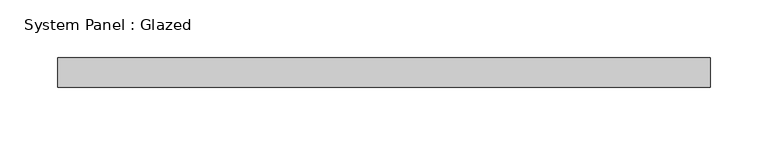
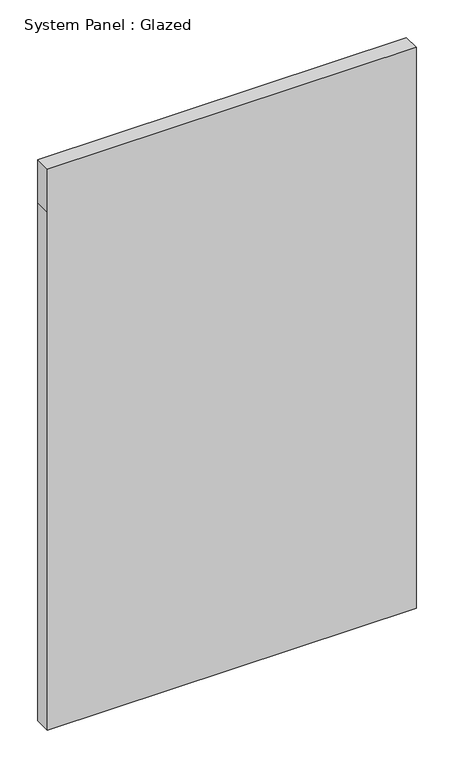
"""IFC4 building model written with IfcOpenShell, lengths in millimetres: plate geometry, System Panel : Glazed."""

from ifc_helpers import new_model, si_unit, frame, origin, place, context, project, spatial, polyline, outline, extrude, source, transform, mapped, element, save


def system_panel_glazed_cdc3472a(model_context):
    return source(origin(), model_context, "Body", "SweptSolid", [
        extrude(outline(polyline([(0.0, -282.575), (0.0, 282.575), (839.0301773, 282.575), (908.8801773, 282.575), (908.8801773, -282.575), (839.0301773, -282.575), (0.0, -282.575)])), frame((0.0, 19.05, 0.0), z_axis=(0.0, 1.0, 0.0), x_axis=(0.0, 0.0, 1.0)), (0.0, 0.0, 1.0), 25.4),
    ])


if __name__ == "__main__":
    model = new_model("IFC4")
    model_context = context("Model", 3, world=origin())
    ifc_project = project(units=[si_unit("LENGTHUNIT", "METRE", prefix="MILLI")], contexts=[model_context])
    site = spatial("IfcSite", under=ifc_project)
    building = spatial("IfcBuilding", under=site)
    placement = place(None, origin())
    system_panel_glazed_shape = system_panel_glazed_cdc3472a(model_context)
    element("IfcPlate", 1, ObjectType="System Panel : Glazed", at=placement, inside=building, context=model_context, shape_type="MappedRepresentation", body=[
        mapped(system_panel_glazed_shape, transform((0.0, 0.0, 0.0), x_axis=(1.0, 0.0, 0.0), y_axis=(0.0, 1.0, 0.0), z_axis=(0.0, 0.0, 1.0))),
    ])
    save(model, "model.ifc")

# Revit data of these elements
# Type "System Panel : Glazed"
#   Construction Type Id = "GSP4R"
#   Analytic Construction = "1/8 in Pilkington single glazing"
#   Visual Light Transmittance = 0.9
#   Solar Heat Gain Coefficient = 0.86
#   Heat Transfer Coefficient (U) = 1.18115 BTU/(h·ft²·°F)
#   Define Thermal Properties by = 1
# Element 1 (IfcPlate, "System Panel : Glazed")
#   Materials on its faces: "Glass"
# Materials
#   "Glass": class "Glass", colour RGB 0 128 192, transparency 0.75, Description = "Soda Lime Glass", Cost = 0
